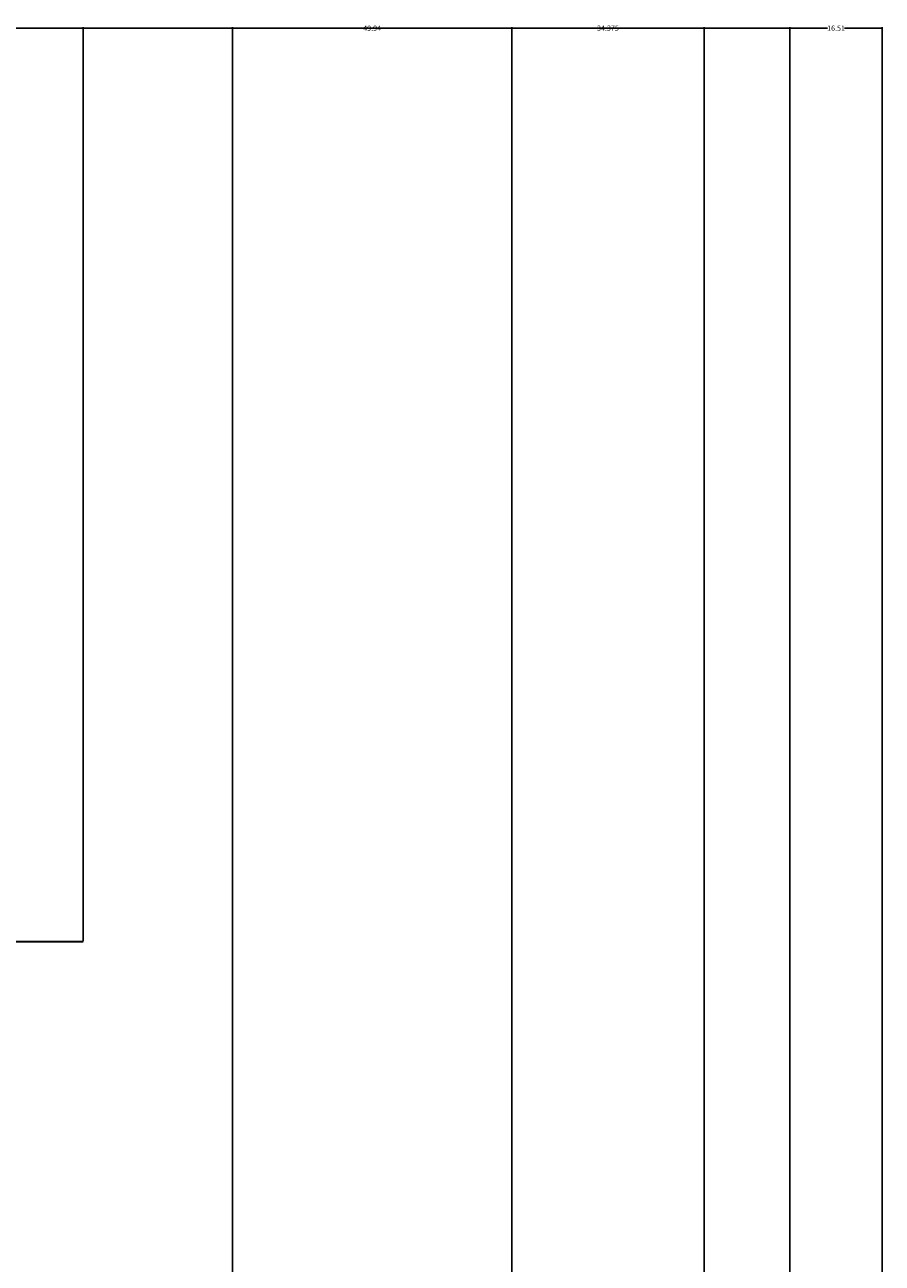
# Model space of a CAD drawing. Units: inches. Extents: x -5 to 714, y 84 to 644.
# Tile 20 of 20: x 457 to 610, y 423 to 644. Entities that reach past the tile are written whole.
import ezdxf

# ---------------------------------------------------------------- set-up
doc = ezdxf.new("R2010")
doc.units = ezdxf.units.IN
doc.header["$MEASUREMENT"] = 0
doc.layers.add('A-ANNO-DIMS', color=2, linetype='Continuous', lineweight=18)
doc.layers.add('A-ELEV', color=7, linetype='Continuous', lineweight=35)
doc.styles.get("Standard").update_dxf_attribs({"font": 'arial.ttf'})
doc.dimstyles.get("Standard").update_dxf_attribs({"dimtxt": 0.9375, "dimasz": 0.18, "dimexe": 0.18, "dimexo": 0.0625, "dimgap": 0.09, "dimtad": 0, "dimtih": 1, "dimtoh": 1, "dimdec": 4, "dimzin": 0, "dimdsep": 46, "dimlunit": 4, "dimtxsty": 'Standard', "dimcen": 0.09, "dimadec": 0, "dimazin": 0, "dimtfac": 1, "dimtdec": 4, "dimtofl": 0, "dimtmove": 0, "dimatfit": 3, "dimfxl": 1, "dimtolj": 1, "dimtzin": 0, "dimarcsym": 0})

# ---------------------------------------------------------------- blocks, each defined once
blk = doc.blocks.new('*D24')
at = {"layer": 'A-ANNO-DIMS', "color": 0, "lineweight": -2, "transparency": 16777216}
for p, q in [((126.73, 480.23), (126.73, 643.61)), ((126.91, 643.43), (295.25, 643.43)), ((466.92, 643.43), (298.58, 643.43)), ((467.1, 480.23), (467.1, 643.61))]:
    blk.add_line(p, q, dxfattribs=at)
at = {"layer": 'A-ANNO-DIMS', "color": 0, "transparency": 16777216}
for points in [[(126.91, 643.46), (126.91, 643.4), (126.73, 643.43)], [(466.92, 643.46), (466.92, 643.4), (467.1, 643.43)]]:
    blk.add_solid(points, dxfattribs=at)
at = {"layer": 'Defpoints', "color": 0, "transparency": 16777216}
for p in [(467.1, 643.43), (126.73, 480.17), (467.1, 480.17)]:
    blk.add_point(p, dxfattribs=at)
at = {"layer": 'A-ANNO-DIMS', "color": 0, "transparency": 16777216, "insert": (296.91, 643.43), "char_height": 0.938, "attachment_point": 5}
blk.add_mtext('\\A1;340.4', dxfattribs=at)
blk = doc.blocks.new('*D54')
at = {"layer": 'A-ANNO-DIMS', "color": 0, "lineweight": -2, "transparency": 16777216}
for p, q in [((259.07, 315.16), (259.07, 643.61)), ((259.25, 643.43), (424.21, 643.43)), ((593.25, 643.43), (428.28, 643.43)), ((593.43, 315.16), (593.43, 643.61))]:
    blk.add_line(p, q, dxfattribs=at)
at = {"layer": 'A-ANNO-DIMS', "color": 0, "transparency": 16777216}
for points in [[(259.25, 643.46), (259.25, 643.4), (259.07, 643.43)], [(593.25, 643.46), (593.25, 643.4), (593.43, 643.43)]]:
    blk.add_solid(points, dxfattribs=at)
at = {"layer": 'Defpoints', "color": 0, "transparency": 16777216}
for p in [(593.43, 643.43), (259.07, 315.1), (593.43, 315.1)]:
    blk.add_point(p, dxfattribs=at)
at = {"layer": 'A-ANNO-DIMS', "color": 0, "transparency": 16777216, "insert": (426.25, 643.43), "char_height": 0.938, "attachment_point": 5}
blk.add_mtext('\\A1;334.36', dxfattribs=at)
blk = doc.blocks.new('*D58')
at = {"layer": 'A-ANNO-DIMS', "color": 0, "lineweight": -2, "transparency": 16777216}
for p, q in [((593.43, 282.26), (593.43, 643.61)), ((593.61, 643.43), (600.15, 643.43)), ((609.76, 643.43), (603.22, 643.43)), ((609.94, 282.26), (609.94, 643.61))]:
    blk.add_line(p, q, dxfattribs=at)
at = {"layer": 'A-ANNO-DIMS', "color": 0, "transparency": 16777216}
for points in [[(593.61, 643.46), (593.61, 643.4), (593.43, 643.43)], [(609.76, 643.46), (609.76, 643.4), (609.94, 643.43)]]:
    blk.add_solid(points, dxfattribs=at)
at = {"layer": 'Defpoints', "color": 0, "transparency": 16777216}
for p in [(609.94, 643.43), (593.43, 282.2), (609.94, 282.2)]:
    blk.add_point(p, dxfattribs=at)
at = {"layer": 'A-ANNO-DIMS', "color": 0, "transparency": 16777216, "insert": (601.68, 643.43), "char_height": 0.938, "attachment_point": 5}
blk.add_mtext('\\A1;16.51', dxfattribs=at)
blk = doc.blocks.new('*D62')
at = {"layer": 'A-ANNO-DIMS', "color": 0, "lineweight": -2, "transparency": 16777216}
for p, q in [((407.38, 266.06), (407.38, 643.61)), ((407.56, 643.43), (449.27, 643.43)), ((493.6, 643.43), (451.89, 643.43)), ((493.78, 266.06), (493.78, 643.61))]:
    blk.add_line(p, q, dxfattribs=at)
at = {"layer": 'A-ANNO-DIMS', "color": 0, "transparency": 16777216}
for points in [[(407.56, 643.46), (407.56, 643.4), (407.38, 643.43)], [(493.6, 643.46), (493.6, 643.4), (493.78, 643.43)]]:
    blk.add_solid(points, dxfattribs=at)
at = {"layer": 'Defpoints', "color": 0, "transparency": 16777216}
for p in [(493.78, 643.43), (407.38, 266), (493.78, 266)]:
    blk.add_point(p, dxfattribs=at)
at = {"layer": 'A-ANNO-DIMS', "color": 0, "transparency": 16777216, "insert": (450.58, 643.43), "char_height": 0.938, "attachment_point": 5}
blk.add_mtext('\\A1;86.4', dxfattribs=at)
blk = doc.blocks.new('*D63')
at = {"layer": 'A-ANNO-DIMS', "color": 0, "lineweight": -2, "transparency": 16777216}
for p, q in [((493.78, 266.06), (493.78, 643.61)), ((493.96, 643.43), (517.06, 643.43)), ((543.54, 643.43), (520.44, 643.43)), ((543.72, 266.06), (543.72, 643.61))]:
    blk.add_line(p, q, dxfattribs=at)
at = {"layer": 'A-ANNO-DIMS', "color": 0, "transparency": 16777216}
for points in [[(493.96, 643.46), (493.96, 643.4), (493.78, 643.43)], [(543.54, 643.46), (543.54, 643.4), (543.72, 643.43)]]:
    blk.add_solid(points, dxfattribs=at)
at = {"layer": 'Defpoints', "color": 0, "transparency": 16777216}
for p in [(543.72, 643.43), (493.78, 266), (543.72, 266)]:
    blk.add_point(p, dxfattribs=at)
at = {"layer": 'A-ANNO-DIMS', "color": 0, "transparency": 16777216, "insert": (518.75, 643.43), "char_height": 0.938, "attachment_point": 5}
blk.add_mtext('\\A1;49.94', dxfattribs=at)
blk = doc.blocks.new('*D64')
at = {"layer": 'A-ANNO-DIMS', "color": 0, "lineweight": -2, "transparency": 16777216}
for p, q in [((543.72, 266.06), (543.72, 643.61)), ((543.9, 643.43), (558.86, 643.43)), ((577.91, 643.43), (562.94, 643.43)), ((578.09, 277.11), (578.09, 643.61))]:
    blk.add_line(p, q, dxfattribs=at)
at = {"layer": 'A-ANNO-DIMS', "color": 0, "transparency": 16777216}
for points in [[(543.9, 643.46), (543.9, 643.4), (543.72, 643.43)], [(577.91, 643.46), (577.91, 643.4), (578.09, 643.43)]]:
    blk.add_solid(points, dxfattribs=at)
at = {"layer": 'Defpoints', "color": 0, "transparency": 16777216}
for p in [(578.09, 643.43), (578.09, 277.05), (543.72, 266)]:
    blk.add_point(p, dxfattribs=at)
at = {"layer": 'A-ANNO-DIMS', "color": 0, "transparency": 16777216, "insert": (560.9, 643.43), "char_height": 0.938, "attachment_point": 5}
blk.add_mtext('\\A1;34.375', dxfattribs=at)

msp = doc.modelspace()

# ---------------------------------------------------------------- linework, layer by layer
at = {"layer": 'A-ELEV'}
msp.add_line((229.3575, 480.1709), (467.0994, 480.1709), dxfattribs=at)

# ---------------------------------------------------------------- dimensions: what is measured, and where the dimension line sits
at = {"layer": 'A-ANNO-DIMS'}
for base, p1, p2, override, picture, middle in [((467.0994, 643.4276), (126.7303, 480.1709), (467.0994, 480.1709), {"dimdec": 1, "dimlfac": 1, "dimrnd": 0, "dimzin": 0, "dimdsep": 46, "dimlunit": 2}, '*D24', (296.9148, 643.4276)), ((593.428, 643.4276), (259.0665, 315.0968), (593.428, 315.0968), {"dimdec": 2, "dimlfac": 1, "dimrnd": 0, "dimzin": 0, "dimdsep": 46, "dimlunit": 2}, '*D54', (426.2472, 643.4276)), ((493.7771, 643.4276), (407.3813, 266.0021), (493.7771, 266.0021), {"dimdec": 1, "dimlfac": 1, "dimrnd": 0, "dimzin": 0, "dimdsep": 46, "dimlunit": 2}, '*D62', (450.5792, 643.4276)), ((543.7164, 643.4276), (493.7771, 266.0021), (543.7164, 266.0021), {"dimdec": 2, "dimlfac": 1, "dimrnd": 0, "dimzin": 0, "dimdsep": 46, "dimlunit": 2}, '*D63', (518.7468, 643.4276)), ((578.0915, 643.4276), (543.7164, 266.0021), (578.0915, 277.0513), {"dimdec": 3, "dimlfac": 1, "dimrnd": 0, "dimzin": 0, "dimdsep": 46, "dimlunit": 2}, '*D64', (560.904, 643.4276)), ((609.9384, 643.4276), (593.428, 282.1969), (609.9384, 282.1969), {"dimdec": 2, "dimlfac": 1, "dimrnd": 0, "dimzin": 0, "dimdsep": 46, "dimlunit": 2}, '*D58', (601.6832, 643.4276))]:
    dim = msp.add_linear_dim(base=base, p1=p1, p2=p2, dimstyle='Standard', override=override, dxfattribs=at)
    dim.commit()
    dim.dimension.update_dxf_attribs({"geometry": picture, "text_midpoint": middle})

doc.saveas('drawing.dxf')
